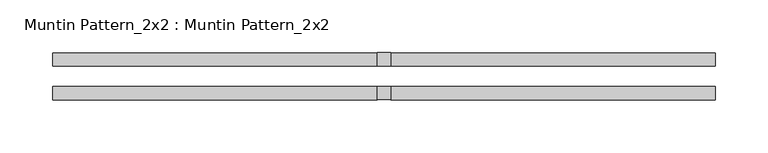
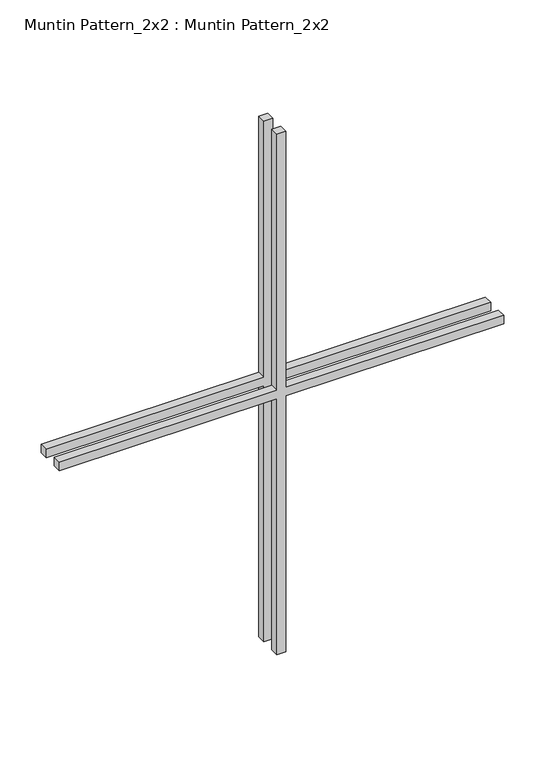
"""IFC4 building model written with IfcOpenShell, lengths in millimetres: proxy geometry, Muntin Pattern_2x2 : Muntin Pattern_2x2."""

from ifc_helpers import new_model, si_unit, frame, origin, place, context, project, spatial, polyline, outline, extrude, source, transform, mapped, element, save


def muntin_pattern_2x2_muntin_pattern_2x2_5c2cbe28(model_context):
    return source(origin(), model_context, "Body", "SweptSolid", [
        extrude(outline(polyline([(393.7, -6.35), (393.7, -312.7375), (381.0, -312.7375), (381.0, -6.35), (0.0, -6.35), (0.0, 6.35), (381.0, 6.35), (381.0, 312.7375), (393.7, 312.7375), (393.7, 6.35), (774.7, 6.35), (774.7, -6.35), (393.7, -6.35)])), frame((0.0, -22.225, 0.0), z_axis=(0.0, 1.0, 0.0), x_axis=(0.0, 0.0, 1.0)), (0.0, 0.0, 1.0), 12.7),
        extrude(outline(polyline([(393.7, -6.35), (393.7, -312.7375), (381.0, -312.7375), (381.0, -6.35), (0.0, -6.35), (0.0, 6.35), (381.0, 6.35), (381.0, 312.7375), (393.7, 312.7375), (393.7, 6.35), (774.7, 6.35), (774.7, -6.35), (393.7, -6.35)])), frame((0.0, 9.525, 0.0), z_axis=(0.0, 1.0, 0.0), x_axis=(0.0, 0.0, 1.0)), (0.0, 0.0, 1.0), 12.7),
    ])


if __name__ == "__main__":
    model = new_model("IFC4")
    model_context = context("Model", 3, world=origin())
    ifc_project = project(units=[si_unit("LENGTHUNIT", "METRE", prefix="MILLI")], contexts=[model_context])
    site = spatial("IfcSite", under=ifc_project)
    building = spatial("IfcBuilding", under=site)
    placement = place(None, origin())
    muntin_pattern_2x2_muntin_pattern_2x2_shape = muntin_pattern_2x2_muntin_pattern_2x2_5c2cbe28(model_context)
    element("IfcBuildingElementProxy", 1, Name="Muntin Pattern_2x2 : Muntin Pattern_2x2", ObjectType="Muntin Pattern_2x2 : Muntin Pattern_2x2", at=placement, inside=building, context=model_context, shape_type="MappedRepresentation", body=[
        mapped(muntin_pattern_2x2_muntin_pattern_2x2_shape, transform((0.0, 0.0, 0.0), x_axis=(1.0, 0.0, 0.0), y_axis=(0.0, 1.0, 0.0), z_axis=(0.0, 0.0, 1.0))),
    ])
    save(model, "model.ifc")

# Revit data of these elements
# Type "Muntin Pattern_2x2 : Muntin Pattern_2x2"
#   Width [instance default] = 4' - 0"
#   Thickness = 0' - 0 1/2"
#   Height [instance default] = 4' - 0"
#   Distance = 0' - 0 3/4"
#   Interior Material [instance default] = none
#   Exterior Material [instance default] = none
#   Default Elevation = 0
# Element 1 (IfcBuildingElementProxy, "Muntin Pattern_2x2 : Muntin Pattern_2x2")
#   Width = 2' - 0 5/8"
#   Height = 2' - 6 1/2"
#   Interior Material = Wood - Stained
#   Exterior Material = Clad - White
#   Materials on its faces: "Clad - White", "Wood - Stained"
# Materials
#   "Clad - White": class "Wood", colour RGB 242 242 238, transparency 0, Cost = 0
#   "Wood - Stained": class "Wood", colour RGB 224 178 126, transparency 0, Cost = 0
